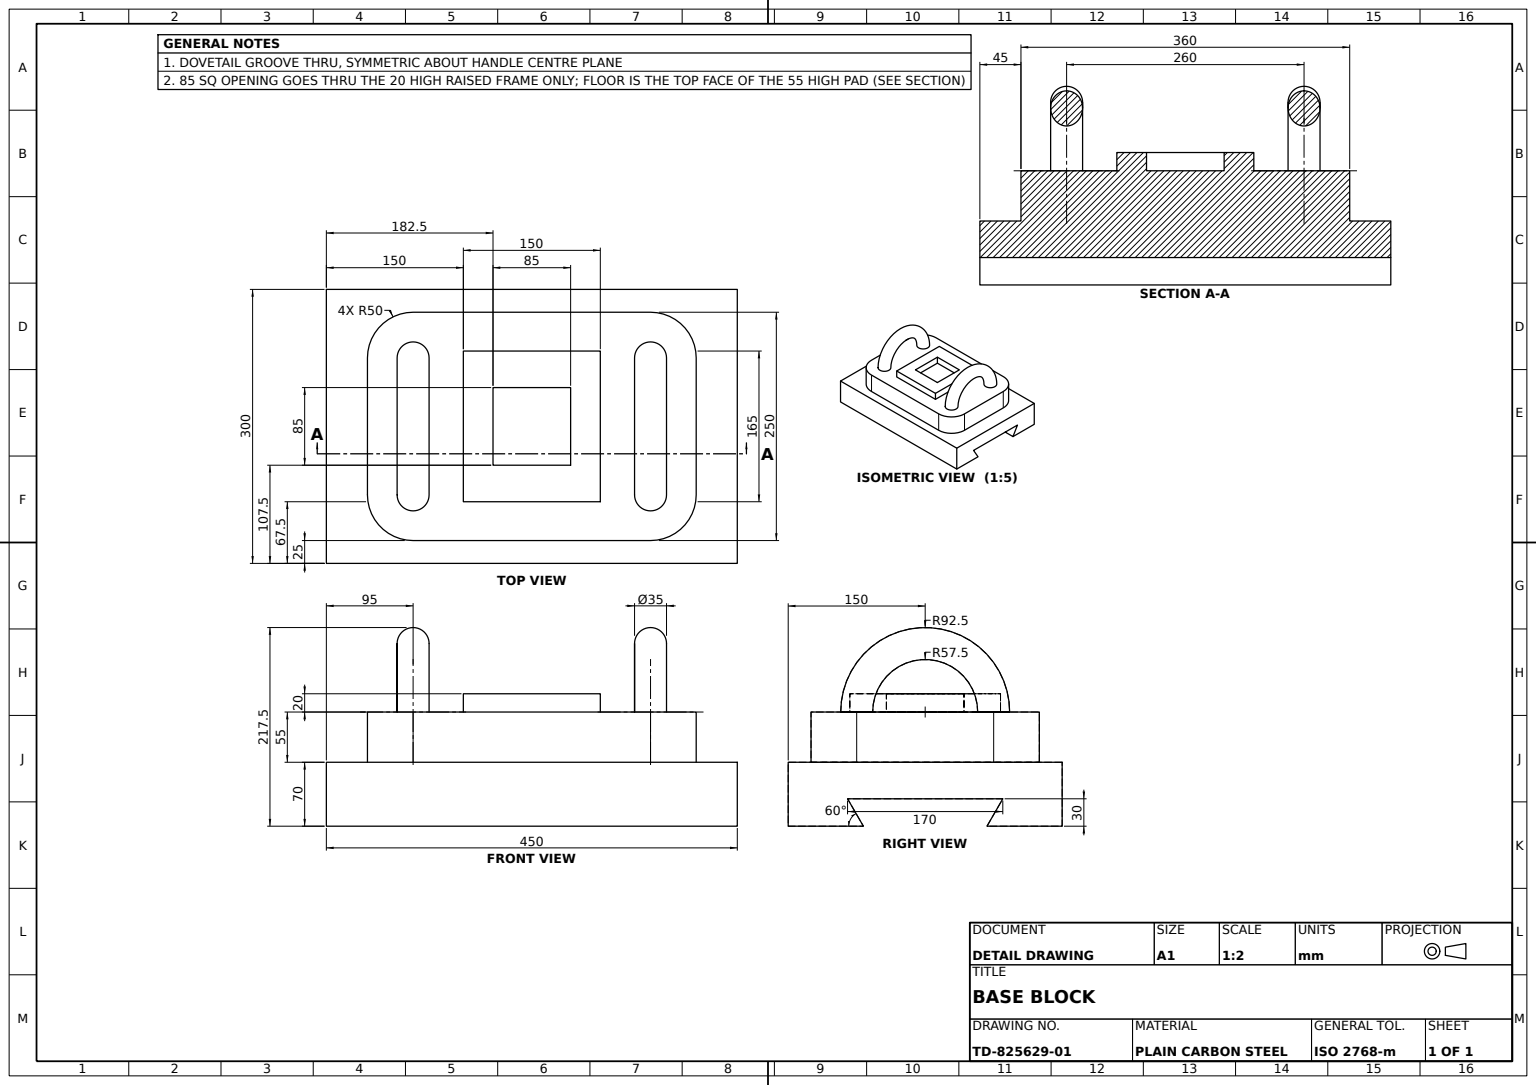
SolidWorks part; units mm, degrees
material "Plain Carbon Steel"
ref_plane "Front Plane" through (0, 0, 0) normal (0, 0, 1) x (1, 0, 0)
ref_plane "Top Plane" through (0, 0, 0) normal (0, 1, 0) x (1, 0, 0)
ref_plane "Right Plane" through (0, 0, 0) normal (1, 0, 0) x (0, 0, -1)
sketch "Base V-Groove Profile Sketch" plane through (0, 0, 0) normal (1, 0, 0) x (0, 0, -1)
  line L0 (-67.6795, 0) -> (-85, 30)
  line L1 (-150, 70) -> (150, 70)
  line L2 (-150, 70) -> (-150, 0)
  line L3 (-150, 0) -> (-67.6795, 0)
  line L4 (150, 70) -> (150, 0)
  line L5 (-85, 30) -> (85, 30)
  line L6 (85, 30) -> (67.6795, 0)
  line L7 (0, 0) -> (0, 29.3993) construction
  line L8 (67.6795, 0) -> (150, 0)
  point P4 (0, 70)
  dimension "D1" = 300
  dimension "D2" = 70
  dimension "D3" = 60
  dimension "D4" = 30
  dimension "D5" = 170
extrude "Base Block V-Groove" add sketch "Base V-Groove Profile Sketch" along normal mid plane 450
sketch "Top Pad Sketch 360x250" plane through (0, 70, 0) normal (0, 1, 0) x (1, 0, 0)
  line L1 (-130, -125) -> (130, -125)
  line L2 (-180, -75) -> (-180, 75)
  line L3 (-130, 125) -> (130, 125)
  line L4 (180, -75) -> (180, 75)
  line L5 (-180, -125) -> (180, 125) construction
  line L6 (-180, 125) -> (180, -125) construction
  arc A0 (-130, -125) -> (-180, -75) centre (-130, -75) cw
  arc A1 (130, -125) -> (180, -75) centre (130, -75) ccw
  arc A2 (130, 125) -> (180, 75) centre (130, 75) cw
  arc A3 (-180, 75) -> (-130, 125) centre (-130, 75) cw
  point P0 (0, 0)
  dimension "D1" = 50
  dimension "D2" = 360
  dimension "D3" = 250
extrude "Top Pad 360x250" add sketch "Top Pad Sketch 360x250" along normal blind 55
sketch "Square Frame Sketch 150" plane through (0, 125, 0) normal (0, 1, 0) x (1, 0, 0)
  line L1 (-75, -82.5) -> (75, -82.5)
  line L2 (-75, -82.5) -> (-75, 82.5)
  line L3 (-75, 82.5) -> (75, 82.5)
  line L4 (75, -82.5) -> (75, 82.5)
  line L5 (-75, -82.5) -> (75, 82.5) construction
  line L6 (-75, 82.5) -> (75, -82.5) construction
  line L7 (-42.5, -42.5) -> (42.5, -42.5)
  line L8 (-42.5, -42.5) -> (-42.5, 42.5)
  line L9 (-42.5, 42.5) -> (42.5, 42.5)
  line L10 (42.5, -42.5) -> (42.5, 42.5)
  line L11 (-42.5, -42.5) -> (42.5, 42.5) construction
  line L12 (-42.5, 42.5) -> (42.5, -42.5) construction
  point P0 (0, 0)
  point P6 (0, 0)
  dimension "D1" = 150
  dimension "D2" = 165
  dimension "D3" = 85
  dimension "D4" = 85
extrude "Square Frame Boss 150" add sketch "Square Frame Sketch 150" along normal blind 20
ref_plane "Handle Path Plane" through (130, 0, 0) normal (1, 0, 0) x (0, 0, -1)
sketch "Handle Path Sketch" plane through (130, 0, 0) normal (1, 0, 0) x (0, 0, -1)
  line L1 (-82.5, 125) -> (82.5, 125) construction
  line L2 (-75, 125) -> (75, 125) construction
  arc A0 (-75, 125) -> (75, 125) centre (0, 125) cw
  dimension "D1" = 150
sweep "Lifting Handle Ø35" add path "Handle Path Sketch" circular profile diameter 35 parameters "D3"=35
mirror "Lifting Handle Mirror" about plane through (0, 0, 0) normal (1, 0, 0) of "Lifting Handle Ø35"
